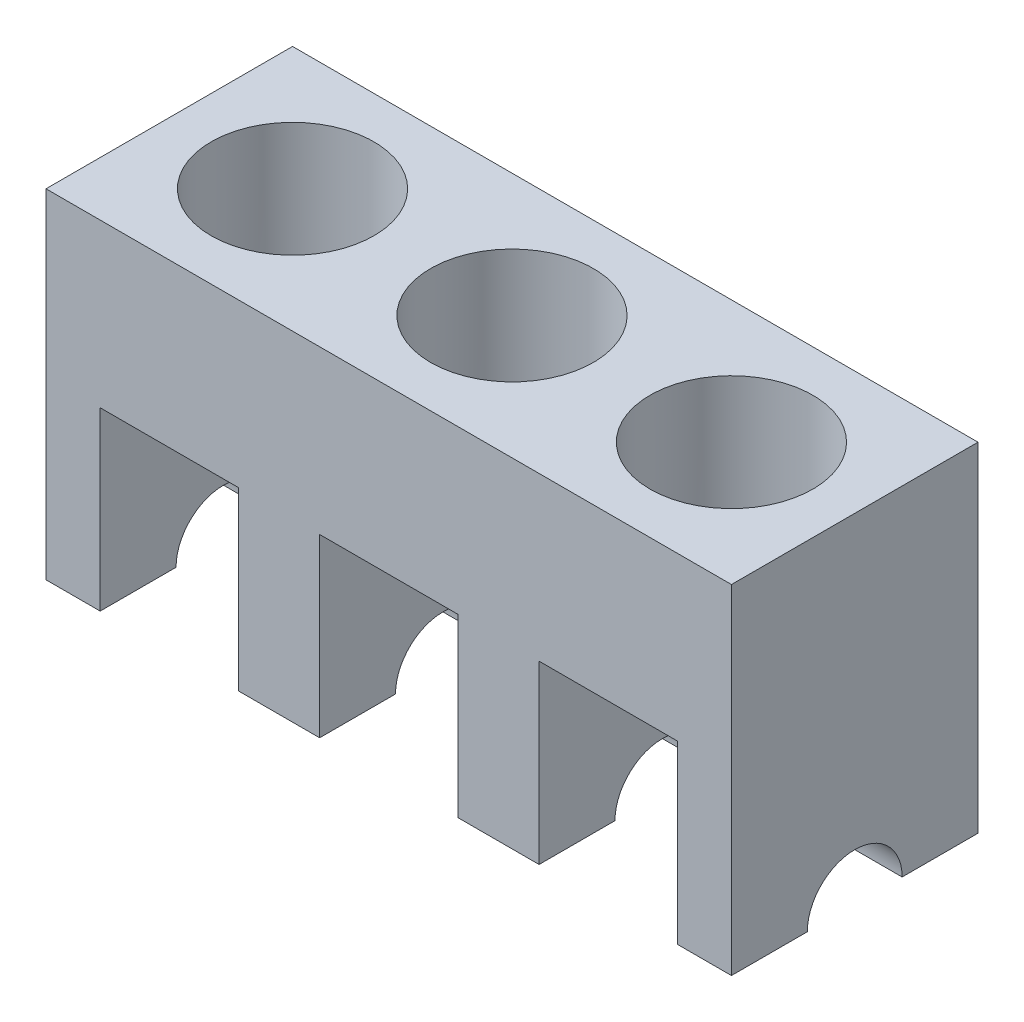
from build123d import *

# Parameters (mm, degrees)
BLOCK_BODY_DEPTH             = 45.5
CRANKSHAFT_BORE_SKETCH_R     = 17.5
CRANKSHAFT_BORE_35_DEPTH     = 265.547727263
CYLINDER_BORES_SKETCH_R      = 30.05
CYLINDER_BORES_3X_45_5_DEPTH = 81


with BuildPart() as part:
    # Block Profile Sketch → Block Body (new, symmetric)
    with BuildSketch(Plane.XY):
        Polygon((-106.5, -62.5), (-106.5, 2.5), (-55.5, 2.5), (-55.5, -62.5), (-25.5, -62.5), (-25.5, 2.5), (25.5, 2.5), (25.5, -62.5), (55.5, -62.5), (55.5, 2.5), (106.5, 2.5), (106.5, -62.5), (126.5, -62.5), (126.5, 62.5), (-126.5, 62.5), (-126.5, -62.5), align=None)
    extrude(amount=BLOCK_BODY_DEPTH, both=True)

    # Crankshaft Bore Sketch → Crankshaft Bore Ø35 (cut, through all)
    with BuildSketch(Plane(origin=(126.5, 0, 0), x_dir=(0, 0, -1), z_dir=(1, 0, 0))):
        with Locations((0, -62.5)):
            Circle(CRANKSHAFT_BORE_SKETCH_R)
    extrude(amount=-CRANKSHAFT_BORE_35_DEPTH, mode=Mode.SUBTRACT)

    # Cylinder Bores Sketch → Cylinder Bores 3xØ45.5 (cut)
    with BuildSketch(Plane(origin=(0, 62.5, 0), x_dir=(1, 0, 0), z_dir=(0, 1, 0))):
        with Locations(Location((-81, 0, 0), (0, 0, 270))):
            Circle(CYLINDER_BORES_SKETCH_R)
        with Locations(Location((0, 0, 0), (0, 0, 270))):
            Circle(CYLINDER_BORES_SKETCH_R)
        with Locations(Location((81, 0, 0), (0, 0, 270))):
            Circle(CYLINDER_BORES_SKETCH_R)
    extrude(amount=-CYLINDER_BORES_3X_45_5_DEPTH, mode=Mode.SUBTRACT)


solid = part.part
